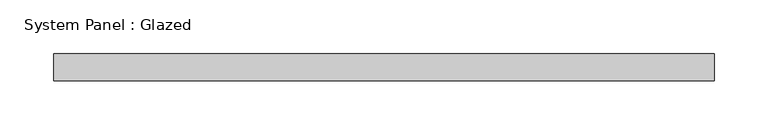
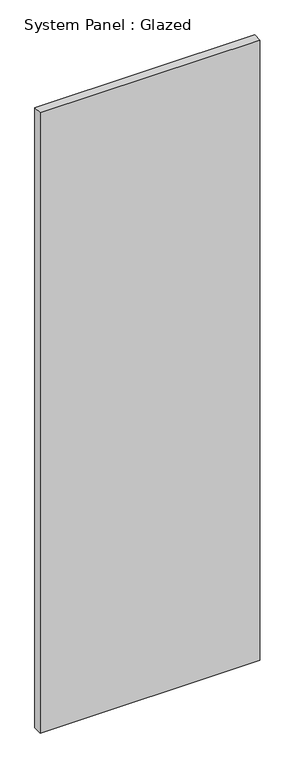
"""IFC4 building model written with IfcOpenShell, lengths in millimetres: plate geometry, System Panel : Glazed."""

from ifc_helpers import new_model, si_unit, origin, origin_with_axes, place, context, project, spatial, polyline, outline, extrude, source, transform, mapped, element, save


def system_panel_glazed_1587745b(model_context):
    return source(origin(), model_context, "Body", "SweptSolid", [
        extrude(outline(polyline([(307.975, 19.05), (-307.975, 19.05), (-307.975, 44.45), (307.975, 44.45), (307.975, 19.05)])), origin_with_axes(), (0.0, 0.0, 1.0), 1837.4891744),
    ])


if __name__ == "__main__":
    model = new_model("IFC4")
    model_context = context("Model", 3, world=origin())
    ifc_project = project(units=[si_unit("LENGTHUNIT", "METRE", prefix="MILLI")], contexts=[model_context])
    site = spatial("IfcSite", under=ifc_project)
    building = spatial("IfcBuilding", under=site)
    placement = place(None, origin())
    system_panel_glazed_shape = system_panel_glazed_1587745b(model_context)
    element("IfcPlate", 1, ObjectType="System Panel : Glazed", at=placement, inside=building, context=model_context, shape_type="MappedRepresentation", body=[
        mapped(system_panel_glazed_shape, transform((0.0, 0.0, 0.0), x_axis=(1.0, 0.0, 0.0), y_axis=(0.0, 1.0, 0.0), z_axis=(0.0, 0.0, 1.0))),
    ])
    save(model, "model.ifc")

# Revit data of these elements
# Type "System Panel : Glazed"
#   Construction Type Id = "GSP4R"
#   Analytic Construction = "1/8 in Pilkington single glazing"
#   Visual Light Transmittance = 0.9
#   Solar Heat Gain Coefficient = 0.86
#   Heat Transfer Coefficient (U) = 1.18115 BTU/(h·ft²·°F)
#   Define Thermal Properties by = 1
# Element 1 (IfcPlate, "System Panel : Glazed")
#   Materials on its faces: "Glass"
# Materials
#   "Glass": class "Glass", colour RGB 0 128 192, transparency 0.75, Description = "Soda Lime Glass", Cost = 0
